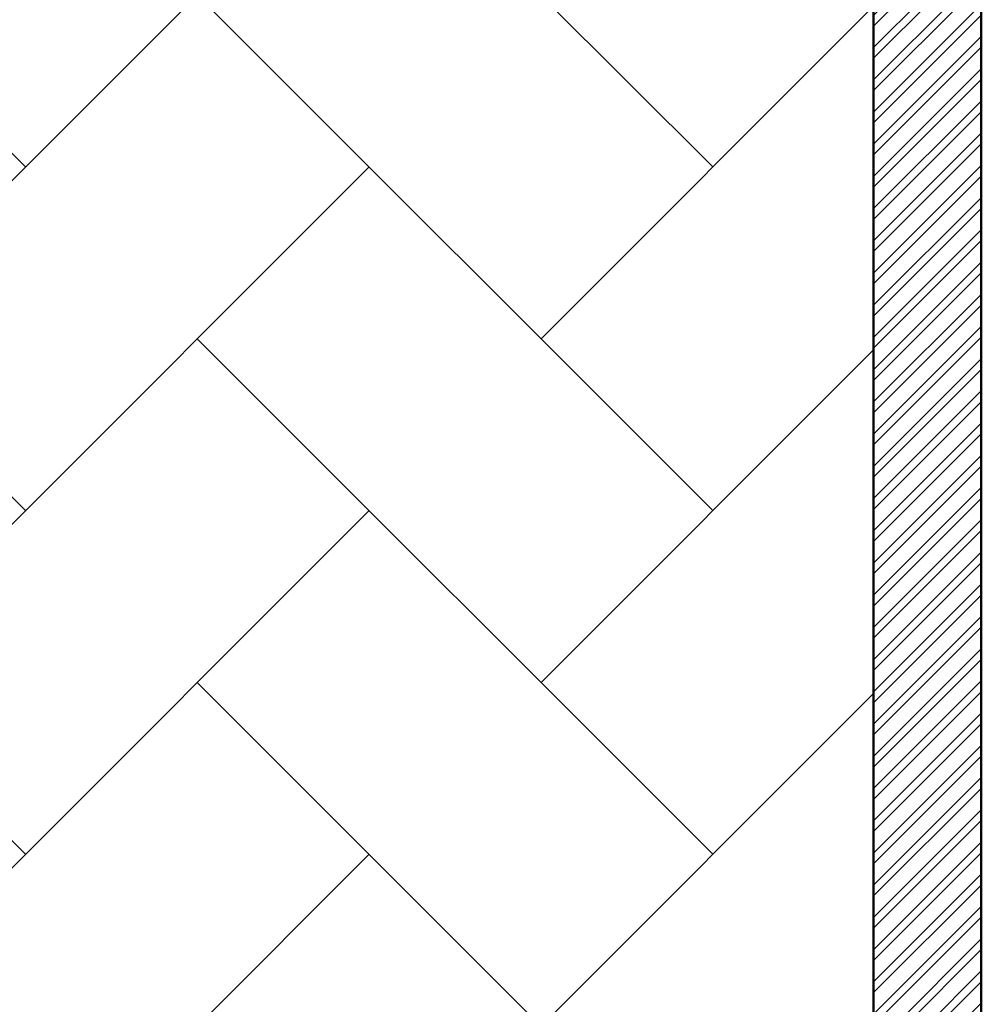
# Model space of a CAD drawing. Units: inches. Extents: x 3590 to 5167, y 65 to 1917.
# Tile 68 of 100: x 5000 to 5080, y 1640 to 1722. Entities that reach past the tile are written whole.
import ezdxf

# ---------------------------------------------------------------- set-up
doc = ezdxf.new("R2010")
doc.units = ezdxf.units.IN
for name, color, linetype, lineweight in [('A-FLOR-PATT', 8, 'Continuous', 13), ('A-WALL', 7, 'Continuous', 50), ('A-WALL-PATT', 251, 'Continuous', 13)]:
    doc.layers.add(name, color=color, linetype=linetype, lineweight=lineweight)

msp = doc.modelspace()

# ---------------------------------------------------------------- hatches: boundary and pattern name
at = {"layer": 'A-FLOR-PATT', "transparency": 33554687}
h = msp.add_hatch(dxfattribs=at)
h.set_pattern_fill('AR-HBONE', color=256, scale=0.2)
h.set_pattern_definition([(45, (-588.972, 0), (0, 28.73682), [60.96, -20.32]), (135, (-574.604, 14.368), (3e-15, 28.73682), [60.96, -20.32])])
h.paths.add_polyline_path([(5071.274, 1796.999), (4933.274, 1796.999), (4933.274, 1753.999), (4962.774, 1753.999, -0.414214), (4928.774, 1719.999), (4933.274, 1718.999), (4933.274, 1334.999), (5071.274, 1334.999)])
h.paths.add_polyline_path([(4951.78, 1521.077), (4951.715, 1521.04), (4951.563, 1520.895)], flags=16)
h.paths.add_polyline_path([(4952.267, 1521.376), (4952.198, 1521.371), (4952.198, 1521.356)], flags=0)
h.paths.add_polyline_path([(4967.051, 1529.728), (4965.231, 1528.694), (4963.411, 1527.714), (4961.756, 1526.851), (4963.589, 1527.449), (4964.036, 1527.478), (4962.975, 1527.249), (4961.76, 1526.852), (4959.792, 1525.834), (4958.005, 1524.895), (4956.24, 1523.93), (4954.504, 1522.919), (4954.129, 1522.682), (4953.361, 1521.997), (4953.366, 1521.998), (4953.605, 1522.064), (4955.106, 1522.761), (4956.921, 1523.434), (4958.678, 1523.915), (4960.358, 1524.2), (4961.945, 1524.286), (4964.171, 1524.108), (4965.958, 1523.309), (4963.863, 1522.976), (4965.187, 1522.499), (4963.366, 1522.497), (4961.545, 1522.487), (4959.764, 1522.461), (4958.304, 1522.419), (4957.974, 1522.388), (4956.307, 1522.232), (4954.718, 1522.071), (4953.251, 1521.899), (4953.525, 1521.623), (4954.331, 1521.379), (4956.243, 1521.23), (4958.039, 1520.93), (4959.684, 1520.483), (4961.16, 1519.896), (4963.107, 1518.8), (4964.393, 1517.325), (4962.973, 1517.726), (4964.558, 1516.661), (4965.407, 1515.708), (4963.507, 1516.322), (4961.68, 1517.005), (4959.935, 1517.745), (4958.282, 1518.528), (4956.732, 1519.343), (4955.295, 1520.175), (4954.672, 1520.572), (4954.513, 1520.627), (4955.658, 1519.318), (4956.703, 1517.982), (4957.644, 1516.647), (4958.485, 1515.334), (4959.55, 1513.524), (4960.438, 1511.769), (4958.841, 1513.62), (4957.452, 1515.325), (4955.819, 1517.459), (4956.665, 1515.448), (4957.111, 1513.923), (4957.447, 1511.714), (4957.076, 1509.793), (4956.538, 1511.11), (4955.992, 1512.569), (4955.444, 1514.125), (4954.898, 1515.735), (4954.357, 1517.356), (4953.824, 1518.943), (4953.305, 1520.452), (4953.065, 1521.116), (4952.971, 1521.146), (4952.949, 1521.086), (4952.73, 1520.199), (4953.37, 1518.024), (4953.757, 1516.373), (4954.051, 1514.765), (4954.264, 1513.221), (4954.471, 1511.131), (4954.497, 1510.402), (4954.409, 1511.76), (4954.264, 1513.221), (4954.051, 1514.765), (4953.757, 1516.373), (4953.37, 1518.024), (4952.877, 1519.698), (4952.716, 1520.141), (4952.533, 1519.059), (4952.374, 1517.789), (4952.219, 1516.312), (4952.046, 1514.6), (4951.833, 1512.626), (4951.557, 1510.363), (4951.203, 1512.168), (4950.852, 1514.339), (4950.985, 1516.376), (4951.66, 1518.286), (4952.593, 1520.481), (4952.357, 1521.13), (4951.855, 1520.328), (4950.839, 1518.908), (4949.777, 1517.587), (4948.916, 1516.617), (4948.111, 1515.256), (4947.089, 1513.554), (4945.889, 1511.615), (4946.326, 1513.402), (4946.562, 1514.249), (4945.528, 1513.327), (4944.581, 1512.531), (4946.018, 1514.508), (4947.204, 1516.048), (4947.893, 1517.313), (4949.307, 1518.764), (4950.414, 1519.767), (4950.451, 1519.806), (4952.267, 1521.376), (4951.645, 1521.493), (4950.404, 1521.18), (4948.044, 1520.359), (4946.119, 1519.452), (4944.572, 1518.475), (4943.35, 1517.443), (4941.997, 1515.92), (4941.661, 1515.275), (4942.813, 1516.99), (4944.572, 1518.475), (4946.119, 1519.452), (4948.044, 1520.359), (4950.404, 1521.18), (4951.645, 1521.493), (4949.647, 1521.868), (4948.6, 1521.756), (4947.126, 1521.57), (4945.42, 1521.348), (4943.45, 1521.105), (4941.183, 1520.856), (4942.86, 1521.613), (4943.873, 1522.03), (4942.952, 1521.909), (4941.41, 1521.485), (4939.543, 1520.67), (4938.968, 1520.226), (4940.733, 1521.299), (4942.952, 1521.909), (4943.702, 1522.008), (4945.894, 1522.7), (4947.565, 1522.714), (4948.921, 1522.566), (4951.131, 1522.183), (4950.971, 1522.297), (4948.129, 1523.006), (4946.035, 1523.707), (4944.232, 1524.521), (4942.707, 1525.461), (4941.444, 1526.537), (4940.43, 1527.761), (4939.649, 1529.143), (4941.421, 1528.122), (4943.147, 1527.132), (4944.841, 1526.175), (4946.514, 1525.25), (4948.179, 1524.359), (4948.365, 1524.263), (4946.475, 1526.045), (4945.181, 1527.54), (4944.19, 1529.033), (4943.496, 1530.54), (4943.278, 1531.36), (4942.498, 1531.919), (4943.114, 1531.762), (4942.959, 1533.659), (4944.14, 1531.989), (4944.612, 1531.323), (4946.202, 1530.463), (4947.486, 1529.509), (4948.79, 1528.226), (4950.368, 1526.237), (4949.485, 1528.155), (4948.851, 1530.123), (4948.491, 1532.041), (4948.381, 1533.918), (4948.501, 1535.76), (4948.827, 1537.573), (4949.418, 1535.565), (4949.957, 1533.569), (4950.464, 1531.586), (4950.961, 1529.617), (4951.391, 1527.954), (4951.724, 1530.687), (4952.201, 1532.58), (4952.889, 1534.33), (4953.77, 1535.951), (4954.827, 1537.46), (4954.521, 1535.39), (4954.273, 1533.937), (4955.58, 1535.663), (4956.748, 1536.739), (4956.159, 1534.78), (4955.589, 1532.873), (4955.043, 1531.006), (4954.525, 1529.166), (4954.038, 1527.341), (4953.638, 1525.733), (4953.611, 1525.586), (4953.398, 1524.166), (4953.382, 1524.009), (4954.07, 1525.476), (4954.912, 1527.022), (4956.136, 1528.894), (4957.847, 1530.577), (4959.376, 1531.54), (4958.256, 1530.104), (4957.143, 1528.663), (4956.066, 1527.243), (4955.056, 1525.871), (4954.141, 1524.571), (4953.352, 1523.372), (4953.311, 1523.303), (4953.273, 1522.925), (4953.261, 1522.382), (4954.103, 1523.373), (4954.63, 1524.284), (4955.961, 1526.358), (4957.23, 1528.13), (4958.421, 1529.609), (4960.037, 1531.368), (4961.374, 1532.375), (4962.101, 1532.77), (4961.07, 1531.061), (4959.987, 1529.438), (4958.869, 1527.908), (4958.15, 1527.007), (4959.803, 1528.003), (4961.589, 1528.793), (4963.391, 1529.328), (4965.211, 1529.632)], flags=16)
h.paths.add_polyline_path([(4962.944, 1523.182), (4961.107, 1523.422), (4960.392, 1523.362), (4962.35, 1523.331)], flags=0)
h.paths.add_polyline_path([(5049.541, 1584.551), (5049.476, 1584.515), (5049.325, 1584.37)], flags=16)
h.paths.add_polyline_path([(5050.028, 1584.851), (5049.959, 1584.845), (5049.959, 1584.83)], flags=0)
h.paths.add_polyline_path([(5042.333, 1581.949), (5043.88, 1582.926), (5045.806, 1583.833), (5048.165, 1584.654), (5049.406, 1584.967), (5047.408, 1585.342), (5046.361, 1585.231), (5044.888, 1585.044), (5043.181, 1584.822), (5041.211, 1584.579), (5038.944, 1584.33), (5040.622, 1585.087), (5041.634, 1585.504), (5040.713, 1585.383), (5039.171, 1584.959), (5037.304, 1584.144), (5036.729, 1583.7), (5038.494, 1584.773), (5040.713, 1585.383), (5041.463, 1585.482), (5043.655, 1586.174), (5045.326, 1586.188), (5046.682, 1586.04), (5048.893, 1585.657), (5048.732, 1585.771), (5045.891, 1586.48), (5043.796, 1587.181), (5041.994, 1587.996), (5040.468, 1588.935), (5039.205, 1590.011), (5038.191, 1591.235), (5037.41, 1592.617), (5039.182, 1591.596), (5040.909, 1590.607), (5042.602, 1589.649), (5044.275, 1588.724), (5045.94, 1587.833), (5046.126, 1587.738), (5044.237, 1589.519), (5042.942, 1591.015), (5041.952, 1592.508), (5041.257, 1594.014), (5041.039, 1594.834), (5040.26, 1595.393), (5040.875, 1595.237), (5040.721, 1597.133), (5041.901, 1595.463), (5042.373, 1594.798), (5043.963, 1593.938), (5045.247, 1592.983), (5046.552, 1591.701), (5048.129, 1589.712), (5047.247, 1591.63), (5046.613, 1593.597), (5046.252, 1595.515), (5046.142, 1597.392), (5046.262, 1599.234), (5046.588, 1601.047), (5047.179, 1599.039), (5047.718, 1597.043), (5048.225, 1595.06), (5048.722, 1593.091), (5049.152, 1591.429), (5049.485, 1594.161), (5049.962, 1596.054), (5050.65, 1597.804), (5051.532, 1599.425), (5052.589, 1600.934), (5052.283, 1598.864), (5052.034, 1597.411), (5053.341, 1599.137), (5054.509, 1600.213), (5053.92, 1598.254), (5053.35, 1596.348), (5052.805, 1594.48), (5052.286, 1592.64), (5051.799, 1590.815), (5051.4, 1589.207), (5051.373, 1589.06), (5051.159, 1587.64), (5051.143, 1587.483), (5051.831, 1588.95), (5052.673, 1590.496), (5053.898, 1592.368), (5055.608, 1594.051), (5057.137, 1595.014), (5056.017, 1593.578), (5054.904, 1592.137), (5053.828, 1590.717), (5052.817, 1589.345), (5051.902, 1588.046), (5051.113, 1586.846), (5051.072, 1586.777), (5051.034, 1586.399), (5051.022, 1585.856), (5051.864, 1586.847), (5052.391, 1587.758), (5053.723, 1589.832), (5054.991, 1591.604), (5056.182, 1593.083), (5057.798, 1594.842), (5059.135, 1595.849), (5059.863, 1596.244), (5058.831, 1594.535), (5057.749, 1592.912), (5056.63, 1591.382), (5055.912, 1590.482), (5057.564, 1591.477), (5059.35, 1592.267), (5061.152, 1592.802), (5062.972, 1593.106), (5064.812, 1593.203), (5062.992, 1592.169), (5061.172, 1591.188), (5059.518, 1590.325), (5061.35, 1590.924), (5061.797, 1590.952), (5060.737, 1590.723), (5059.521, 1590.326), (5057.553, 1589.308), (5055.766, 1588.369), (5054.002, 1587.404), (5052.265, 1586.393), (5051.891, 1586.156), (5051.122, 1585.471), (5051.127, 1585.472), (5051.366, 1585.538), (5052.867, 1586.235), (5054.682, 1586.908), (5056.439, 1587.389), (5058.12, 1587.675), (5059.706, 1587.76), (5061.933, 1587.583), (5063.719, 1586.783), (5061.624, 1586.45), (5062.949, 1585.973), (5061.127, 1585.971), (5059.307, 1585.961), (5057.525, 1585.935), (5056.065, 1585.893), (5055.735, 1585.862), (5054.068, 1585.707), (5052.479, 1585.546), (5051.012, 1585.373), (5051.286, 1585.097), (5052.092, 1584.853), (5054.004, 1584.704), (5055.8, 1584.404), (5057.446, 1583.958), (5058.921, 1583.37), (5060.868, 1582.274), (5062.154, 1580.799), (5060.734, 1581.2), (5062.32, 1580.135), (5063.168, 1579.182), (5061.269, 1579.796), (5059.441, 1580.479), (5057.696, 1581.219), (5056.043, 1582.003), (5054.493, 1582.817), (5053.057, 1583.649), (5052.433, 1584.047), (5052.274, 1584.101), (5053.42, 1582.793), (5054.464, 1581.457), (5055.405, 1580.121), (5056.247, 1578.809), (5057.311, 1576.998), (5058.199, 1575.244), (5056.602, 1577.094), (5055.213, 1578.799), (5053.58, 1580.933), (5054.427, 1578.922), (5054.872, 1577.397), (5055.208, 1575.189), (5054.838, 1573.267), (5054.299, 1574.584), (5053.754, 1576.043), (5053.206, 1577.599), (5052.659, 1579.209), (5052.118, 1580.83), (5051.585, 1582.417), (5051.066, 1583.927), (5050.826, 1584.59), (5050.733, 1584.62), (5050.711, 1584.561), (5050.491, 1583.673), (5051.131, 1581.498), (5051.518, 1579.847), (5051.813, 1578.24), (5052.026, 1576.695), (5052.233, 1574.605), (5052.258, 1573.876), (5052.17, 1575.234), (5052.026, 1576.695), (5051.813, 1578.24), (5051.518, 1579.847), (5051.131, 1581.498), (5050.638, 1583.172), (5050.477, 1583.615), (5050.294, 1582.533), (5050.136, 1581.263), (5049.981, 1579.786), (5049.807, 1578.074), (5049.594, 1576.1), (5049.318, 1573.837), (5048.965, 1575.642), (5048.613, 1577.813), (5048.747, 1579.85), (5049.421, 1581.76), (5050.354, 1583.955), (5050.118, 1584.604), (5049.616, 1583.802), (5048.6, 1582.382), (5047.538, 1581.061), (5046.677, 1580.091), (5045.872, 1578.73), (5044.85, 1577.028), (5043.651, 1575.089), (5044.087, 1576.877), (5044.324, 1577.723), (5043.289, 1576.801), (5042.342, 1576.005), (5043.779, 1577.982), (5044.966, 1579.522), (5045.655, 1580.787), (5047.068, 1582.239), (5048.175, 1583.241), (5048.213, 1583.28), (5050.028, 1584.851), (5049.406, 1584.967), (5048.165, 1584.654), (5045.806, 1583.833), (5043.88, 1582.926), (5042.333, 1581.949), (5041.111, 1580.917), (5039.758, 1579.394), (5039.423, 1578.749), (5040.575, 1580.464)], flags=16)
h.paths.add_polyline_path([(4954.799, 1533.12), (4954.262, 1532.079), (4953.831, 1530.935), (4953.505, 1529.636), (4953.283, 1528.133), (4953.167, 1526.376), (4953.156, 1524.315), (4953.277, 1521.236), (4952.802, 1521.842), (4951.557, 1521.998), (4950.976, 1521.961), (4952.661, 1521.941), (4952.802, 1521.842), (4953.152, 1523.593), (4953.167, 1526.376), (4953.283, 1528.133), (4953.609, 1530.346), (4954.456, 1532.592)], flags=0)
h.paths.add_polyline_path([(5050.563, 1585.316), (5049.318, 1585.472), (5048.737, 1585.435), (5050.422, 1585.415), (5050.563, 1585.316), (5050.914, 1587.067), (5050.928, 1589.851), (5051.045, 1591.607), (5051.371, 1593.82), (5052.217, 1596.066), (5052.56, 1596.594), (5052.024, 1595.554), (5051.592, 1594.409), (5051.266, 1593.11), (5051.045, 1591.607), (5050.928, 1589.851), (5050.918, 1587.789), (5051.038, 1584.71)], flags=0)
h.paths.add_polyline_path([(5058.153, 1586.836), (5060.111, 1586.805), (5060.705, 1586.656), (5058.868, 1586.896)], flags=0)
h.paths.add_polyline_path([(5049.541, 1430.936), (5049.476, 1430.9), (5049.325, 1430.755)], flags=16)
h.paths.add_polyline_path([(5050.028, 1431.236), (5049.959, 1431.231), (5049.959, 1431.215)], flags=0)
h.paths.add_polyline_path([(5046.588, 1447.432), (5047.179, 1445.425), (5047.718, 1443.429), (5048.225, 1441.446), (5048.722, 1439.476), (5049.152, 1437.814), (5049.485, 1440.546), (5049.962, 1442.439), (5050.65, 1444.189), (5051.532, 1445.811), (5052.589, 1447.319), (5052.283, 1445.249), (5052.034, 1443.796), (5053.341, 1445.522), (5054.509, 1446.598), (5053.92, 1444.64), (5053.35, 1442.733), (5052.805, 1440.865), (5052.286, 1439.025), (5051.799, 1437.201), (5051.4, 1435.592), (5051.373, 1435.445), (5051.159, 1434.025), (5051.143, 1433.868), (5051.831, 1435.335), (5052.673, 1436.881), (5053.898, 1438.753), (5055.608, 1440.436), (5057.137, 1441.4), (5056.017, 1439.963), (5054.904, 1438.522), (5053.828, 1437.102), (5052.817, 1435.73), (5051.902, 1434.431), (5051.113, 1433.231), (5051.072, 1433.162), (5051.034, 1432.784), (5051.022, 1432.242), (5051.864, 1433.232), (5052.391, 1434.143), (5053.723, 1436.217), (5054.991, 1437.989), (5056.182, 1439.468), (5057.798, 1441.227), (5059.135, 1442.235), (5059.863, 1442.629), (5058.831, 1440.921), (5057.749, 1439.298), (5056.63, 1437.767), (5055.912, 1436.867), (5057.564, 1437.863), (5059.35, 1438.652), (5061.152, 1439.187), (5062.972, 1439.491), (5064.812, 1439.588), (5062.992, 1438.554), (5061.172, 1437.573), (5059.518, 1436.71), (5061.35, 1437.309), (5061.797, 1437.337), (5060.737, 1437.108), (5059.521, 1436.711), (5057.553, 1435.693), (5055.766, 1434.754), (5054.002, 1433.789), (5052.265, 1432.778), (5051.891, 1432.541), (5051.122, 1431.856), (5051.127, 1431.857), (5051.366, 1431.923), (5052.867, 1432.62), (5054.682, 1433.293), (5056.439, 1433.775), (5058.12, 1434.06), (5059.706, 1434.145), (5061.933, 1433.968), (5063.719, 1433.168), (5061.624, 1432.835), (5062.949, 1432.358), (5061.127, 1432.357), (5059.307, 1432.346), (5057.525, 1432.32), (5056.065, 1432.278), (5055.735, 1432.248), (5054.068, 1432.092), (5052.479, 1431.931), (5051.012, 1431.759), (5051.286, 1431.482), (5052.092, 1431.238), (5054.004, 1431.089), (5055.8, 1430.789), (5057.446, 1430.343), (5058.921, 1429.755), (5060.868, 1428.66), (5062.154, 1427.185), (5060.734, 1427.585), (5062.32, 1426.52), (5063.168, 1425.567), (5061.269, 1426.181), (5059.441, 1426.865), (5057.696, 1427.604), (5056.043, 1428.388), (5054.493, 1429.202), (5053.057, 1430.034), (5052.433, 1430.432), (5052.274, 1430.487), (5053.42, 1429.178), (5054.464, 1427.842), (5055.405, 1426.506), (5056.247, 1425.194), (5057.311, 1423.383), (5058.199, 1421.629), (5056.602, 1423.479), (5055.213, 1425.184), (5053.58, 1427.318), (5054.427, 1425.307), (5054.872, 1423.782), (5055.208, 1421.574), (5054.838, 1419.652), (5054.299, 1420.97), (5053.754, 1422.428), (5053.206, 1423.984), (5052.659, 1425.595), (5052.118, 1427.215), (5051.585, 1428.802), (5051.066, 1430.312), (5050.826, 1430.975), (5050.733, 1431.005), (5050.711, 1430.946), (5050.491, 1430.058), (5051.131, 1427.883), (5051.518, 1426.232), (5051.813, 1424.625), (5052.026, 1423.081), (5052.233, 1420.991), (5052.258, 1420.261), (5052.17, 1421.619), (5052.026, 1423.081), (5051.813, 1424.625), (5051.518, 1426.232), (5051.131, 1427.883), (5050.638, 1429.558), (5050.477, 1430.001), (5050.294, 1428.918), (5050.136, 1427.648), (5049.981, 1426.171), (5049.807, 1424.459), (5049.594, 1422.485), (5049.318, 1420.222), (5048.965, 1422.028), (5048.613, 1424.199), (5048.747, 1426.235), (5049.421, 1428.146), (5050.354, 1430.34), (5050.118, 1430.989), (5049.616, 1430.187), (5048.6, 1428.768), (5047.538, 1427.446), (5046.677, 1426.477), (5045.872, 1425.116), (5044.85, 1423.413), (5043.651, 1421.474), (5044.087, 1423.262), (5044.324, 1424.109), (5043.289, 1423.186), (5042.342, 1422.391), (5043.779, 1424.368), (5044.966, 1425.907), (5045.655, 1427.173), (5047.068, 1428.624), (5048.175, 1429.627), (5048.213, 1429.666), (5050.028, 1431.236), (5049.406, 1431.353), (5048.165, 1431.039), (5045.806, 1430.218), (5043.88, 1429.311), (5042.333, 1428.334), (5041.111, 1427.302), (5039.758, 1425.779), (5039.423, 1425.134), (5040.575, 1426.849), (5042.333, 1428.334), (5043.88, 1429.311), (5045.806, 1430.218), (5048.165, 1431.039), (5049.406, 1431.353), (5047.408, 1431.727), (5046.361, 1431.616), (5044.888, 1431.429), (5043.181, 1431.207), (5041.211, 1430.964), (5038.944, 1430.715), (5040.622, 1431.472), (5041.634, 1431.89), (5040.713, 1431.769), (5039.171, 1431.345), (5037.304, 1430.53), (5036.729, 1430.085), (5038.494, 1431.158), (5040.713, 1431.769), (5041.463, 1431.867), (5043.655, 1432.559), (5045.326, 1432.573), (5046.682, 1432.425), (5048.893, 1432.042), (5048.732, 1432.156), (5045.891, 1432.865), (5043.796, 1433.566), (5041.994, 1434.381), (5040.468, 1435.321), (5039.205, 1436.396), (5038.191, 1437.62), (5037.41, 1439.002), (5039.182, 1437.982), (5040.909, 1436.992), (5042.602, 1436.034), (5044.275, 1435.109), (5045.94, 1434.218), (5046.126, 1434.123), (5044.237, 1435.904), (5042.942, 1437.4), (5041.952, 1438.893), (5041.257, 1440.399), (5041.039, 1441.219), (5040.26, 1441.778), (5040.875, 1441.622), (5040.721, 1443.518), (5041.901, 1441.848), (5042.373, 1441.183), (5043.963, 1440.323), (5045.247, 1439.369), (5046.552, 1438.086), (5048.129, 1436.097), (5047.247, 1438.015), (5046.613, 1439.982), (5046.252, 1441.901), (5046.142, 1443.778), (5046.262, 1445.619)], flags=16)
h.paths.add_polyline_path([(5052.382, 1444.255), (5051.623, 1442.78), (5052.024, 1441.939), (5052.56, 1442.98)], flags=0)
h.paths.add_polyline_path([(5050.563, 1431.701), (5049.318, 1431.857), (5048.737, 1431.821), (5050.422, 1431.8)], flags=0)
h.paths.add_polyline_path([(5058.153, 1433.221), (5060.111, 1433.19), (5060.705, 1433.041), (5058.868, 1433.281)], flags=0)
h.paths.add_polyline_path([(5049.541, 1352.285), (5049.476, 1352.249), (5049.325, 1352.104)], flags=16)
h.paths.add_polyline_path([(5050.028, 1352.585), (5049.959, 1352.58), (5049.959, 1352.564)], flags=0)
h.paths.add_polyline_path([(5046.588, 1368.781), (5047.179, 1366.774), (5047.718, 1364.778), (5048.225, 1362.795), (5048.722, 1360.825), (5049.152, 1359.163), (5049.485, 1361.896), (5049.962, 1363.789), (5050.65, 1365.538), (5051.532, 1367.16), (5052.589, 1368.669), (5052.283, 1366.598), (5052.034, 1365.145), (5053.341, 1366.871), (5054.509, 1367.947), (5053.92, 1365.989), (5053.35, 1364.082), (5052.805, 1362.214), (5052.286, 1360.374), (5051.799, 1358.55), (5051.4, 1356.942), (5051.373, 1356.794), (5051.159, 1355.374), (5051.143, 1355.218), (5051.831, 1356.684), (5052.673, 1358.23), (5053.898, 1360.102), (5055.608, 1361.786), (5057.137, 1362.749), (5056.017, 1361.313), (5054.904, 1359.872), (5053.828, 1358.452), (5052.817, 1357.079), (5051.902, 1355.78), (5051.113, 1354.581), (5051.072, 1354.512), (5051.034, 1354.133), (5051.022, 1353.591), (5051.864, 1354.581), (5052.391, 1355.492), (5053.723, 1357.566), (5054.991, 1359.338), (5056.182, 1360.817), (5057.798, 1362.577), (5059.135, 1363.584), (5059.863, 1363.979), (5058.831, 1362.27), (5057.749, 1360.647), (5056.63, 1359.117), (5055.912, 1358.216), (5057.564, 1359.212), (5059.35, 1360.001), (5061.152, 1360.536), (5062.972, 1360.841), (5064.812, 1360.937), (5062.992, 1359.903), (5061.172, 1358.923), (5059.518, 1358.059), (5061.35, 1358.658), (5061.797, 1358.687), (5060.737, 1358.458), (5059.521, 1358.061), (5057.553, 1357.043), (5055.766, 1356.103), (5054.002, 1355.138), (5052.265, 1354.127), (5051.891, 1353.89), (5051.122, 1353.206), (5051.127, 1353.206), (5051.366, 1353.272), (5052.867, 1353.969), (5054.682, 1354.643), (5056.439, 1355.124), (5058.12, 1355.409), (5059.706, 1355.495), (5061.933, 1355.317), (5063.719, 1354.518), (5061.624, 1354.184), (5062.949, 1353.708), (5061.127, 1353.706), (5059.307, 1353.695), (5057.525, 1353.669), (5056.065, 1353.627), (5055.735, 1353.597), (5054.068, 1353.441), (5052.479, 1353.28), (5051.012, 1353.108), (5051.286, 1352.831), (5052.092, 1352.587), (5054.004, 1352.439), (5055.8, 1352.138), (5057.446, 1351.692), (5058.921, 1351.104), (5060.868, 1350.009), (5062.154, 1348.534), (5060.734, 1348.935), (5062.32, 1347.869), (5063.168, 1346.916), (5061.269, 1347.53), (5059.441, 1348.214), (5057.696, 1348.954), (5056.043, 1349.737), (5054.493, 1350.551), (5053.057, 1351.383), (5052.433, 1351.781), (5052.274, 1351.836), (5053.42, 1350.527), (5054.464, 1349.191), (5055.405, 1347.855), (5056.247, 1346.543), (5057.311, 1344.733), (5058.199, 1342.978), (5056.602, 1344.828), (5055.213, 1346.534), (5053.58, 1348.667), (5054.427, 1346.656), (5054.872, 1345.132), (5055.208, 1342.923), (5054.838, 1341.002), (5054.299, 1342.319), (5053.754, 1343.778), (5053.206, 1345.334), (5052.659, 1346.944), (5052.118, 1348.564), (5051.585, 1350.151), (5051.066, 1351.661), (5050.826, 1352.324), (5050.733, 1352.355), (5050.711, 1352.295), (5050.491, 1351.408), (5051.131, 1349.232), (5051.518, 1347.581), (5051.813, 1345.974), (5052.026, 1344.43), (5052.233, 1342.34), (5052.258, 1341.61), (5052.17, 1342.969), (5052.026, 1344.43), (5051.813, 1345.974), (5051.518, 1347.581), (5051.131, 1349.232), (5050.638, 1350.907), (5050.477, 1351.35), (5050.294, 1350.267), (5050.136, 1348.997), (5049.981, 1347.52), (5049.807, 1345.809), (5049.594, 1343.835), (5049.318, 1341.571), (5048.965, 1343.377), (5048.613, 1345.548), (5048.747, 1347.585), (5049.421, 1349.495), (5050.354, 1351.689), (5050.118, 1352.339), (5049.616, 1351.536), (5048.6, 1350.117), (5047.538, 1348.795), (5046.677, 1347.826), (5045.872, 1346.465), (5044.85, 1344.763), (5043.651, 1342.824), (5044.087, 1344.611), (5044.324, 1345.458), (5043.289, 1344.535), (5042.342, 1343.74), (5043.779, 1345.717), (5044.966, 1347.256), (5045.655, 1348.522), (5047.068, 1349.973), (5048.175, 1350.976), (5048.213, 1351.015), (5050.028, 1352.585), (5049.406, 1352.702), (5048.165, 1352.388), (5045.806, 1351.567), (5043.88, 1350.661), (5042.333, 1349.683), (5041.111, 1348.651), (5039.758, 1347.128), (5039.423, 1346.483), (5040.575, 1348.198), (5042.333, 1349.683), (5043.88, 1350.661), (5045.806, 1351.567), (5048.165, 1352.388), (5049.406, 1352.702), (5047.408, 1353.076), (5046.361, 1352.965), (5044.888, 1352.779), (5043.181, 1352.556), (5041.211, 1352.313), (5038.944, 1352.065), (5040.622, 1352.821), (5041.634, 1353.239), (5040.713, 1353.118), (5039.171, 1352.694), (5037.304, 1351.879), (5036.729, 1351.434), (5038.494, 1352.508), (5040.713, 1353.118), (5041.463, 1353.216), (5043.655, 1353.909), (5045.326, 1353.923), (5046.682, 1353.774), (5048.893, 1353.391), (5048.732, 1353.506), (5045.891, 1354.214), (5043.796, 1354.915), (5041.994, 1355.73), (5040.468, 1356.67), (5039.205, 1357.746), (5038.191, 1358.969), (5037.41, 1360.352), (5039.182, 1359.331), (5040.909, 1358.341), (5042.602, 1357.383), (5044.275, 1356.458), (5045.94, 1355.567), (5046.126, 1355.472), (5044.237, 1357.253), (5042.942, 1358.749), (5041.952, 1360.242), (5041.257, 1361.748), (5041.039, 1362.568), (5040.26, 1363.128), (5040.875, 1362.971), (5040.721, 1364.867), (5041.901, 1363.197), (5042.373, 1362.532), (5043.963, 1361.672), (5045.247, 1360.718), (5046.552, 1359.435), (5048.129, 1357.446), (5047.247, 1359.364), (5046.613, 1361.331), (5046.252, 1363.25), (5046.142, 1365.127), (5046.262, 1366.969)], flags=16)
h.paths.add_polyline_path([(5052.382, 1365.604), (5051.623, 1364.129), (5052.024, 1363.288), (5052.56, 1364.329)], flags=0)
h.paths.add_polyline_path([(4951.78, 1698.041), (4951.715, 1698.005), (4951.563, 1697.859)], flags=16)
h.paths.add_polyline_path([(4952.267, 1698.341), (4952.198, 1698.335), (4952.198, 1698.32)], flags=0)
h.paths.add_polyline_path([(4957.076, 1686.757), (4956.538, 1688.074), (4955.992, 1689.533), (4955.444, 1691.089), (4954.898, 1692.699), (4954.357, 1694.32), (4953.824, 1695.907), (4953.305, 1697.417), (4953.065, 1698.08), (4952.971, 1698.11), (4952.949, 1698.051), (4952.73, 1697.163), (4953.37, 1694.988), (4953.757, 1693.337), (4954.051, 1691.729), (4954.264, 1690.185), (4954.471, 1688.095), (4954.497, 1687.366), (4954.409, 1688.724), (4954.264, 1690.185), (4954.051, 1691.729), (4953.757, 1693.337), (4953.37, 1694.988), (4952.877, 1696.662), (4952.716, 1697.105), (4952.533, 1696.023), (4952.374, 1694.753), (4952.219, 1693.276), (4952.046, 1691.564), (4951.833, 1689.59), (4951.557, 1687.327), (4951.203, 1689.132), (4950.852, 1691.303), (4950.985, 1693.34), (4951.66, 1695.25), (4952.593, 1697.445), (4952.357, 1698.094), (4951.855, 1697.292), (4950.839, 1695.872), (4949.777, 1694.551), (4948.916, 1693.581), (4948.111, 1692.22), (4947.089, 1690.518), (4945.889, 1688.579), (4946.326, 1690.366), (4946.562, 1691.213), (4945.528, 1690.291), (4944.581, 1689.495), (4946.018, 1691.472), (4947.204, 1693.012), (4947.893, 1694.277), (4949.307, 1695.729), (4950.414, 1696.731), (4950.451, 1696.77), (4952.267, 1698.341), (4951.645, 1698.457), (4950.404, 1698.144), (4948.044, 1697.323), (4946.119, 1696.416), (4944.572, 1695.439), (4943.35, 1694.407), (4941.997, 1692.884), (4941.661, 1692.239), (4942.813, 1693.954), (4944.572, 1695.439), (4946.119, 1696.416), (4948.044, 1697.323), (4950.404, 1698.144), (4951.645, 1698.457), (4949.647, 1698.832), (4948.6, 1698.72), (4947.126, 1698.534), (4945.42, 1698.312), (4943.45, 1698.069), (4941.183, 1697.82), (4942.86, 1698.577), (4943.873, 1698.994), (4942.952, 1698.873), (4941.41, 1698.449), (4939.543, 1697.634), (4938.968, 1697.19), (4940.733, 1698.263), (4942.952, 1698.873), (4943.702, 1698.972), (4945.894, 1699.664), (4947.565, 1699.678), (4948.921, 1699.53), (4951.131, 1699.147), (4950.971, 1699.261), (4948.129, 1699.97), (4946.035, 1700.671), (4944.232, 1701.486), (4942.707, 1702.425), (4941.444, 1703.501), (4940.43, 1704.725), (4939.649, 1706.107), (4941.421, 1705.086), (4943.147, 1704.097), (4944.841, 1703.139), (4946.514, 1702.214), (4948.179, 1701.323), (4948.365, 1701.227), (4946.475, 1703.009), (4945.181, 1704.505), (4944.19, 1705.997), (4943.496, 1707.504), (4943.278, 1708.324), (4942.498, 1708.883), (4943.114, 1708.727), (4942.959, 1710.623), (4944.14, 1708.953), (4944.612, 1708.287), (4946.202, 1707.428), (4947.486, 1706.473), (4948.79, 1705.191), (4950.368, 1703.202), (4949.485, 1705.12), (4948.851, 1707.087), (4948.491, 1709.005), (4948.381, 1710.882), (4948.501, 1712.724), (4948.827, 1714.537), (4949.418, 1712.529), (4949.957, 1710.533), (4950.464, 1708.55), (4950.961, 1706.581), (4951.391, 1704.919), (4951.724, 1707.651), (4952.201, 1709.544), (4952.889, 1711.294), (4953.77, 1712.915), (4954.827, 1714.424), (4954.521, 1712.354), (4954.273, 1710.901), (4955.58, 1712.627), (4956.748, 1713.703), (4956.159, 1711.744), (4955.589, 1709.837), (4955.043, 1707.97), (4954.525, 1706.13), (4954.038, 1704.305), (4953.638, 1702.697), (4953.611, 1702.55), (4953.398, 1701.13), (4953.382, 1700.973), (4954.07, 1702.44), (4954.912, 1703.986), (4956.136, 1705.858), (4957.847, 1707.541), (4959.376, 1708.504), (4958.256, 1707.068), (4957.143, 1705.627), (4956.066, 1704.207), (4955.056, 1702.835), (4954.141, 1701.536), (4953.352, 1700.336), (4953.311, 1700.267), (4953.273, 1699.889), (4953.261, 1699.346), (4954.103, 1700.337), (4954.63, 1701.248), (4955.961, 1703.322), (4957.23, 1705.094), (4958.421, 1706.573), (4960.037, 1708.332), (4961.374, 1709.339), (4962.101, 1709.734), (4961.07, 1708.025), (4959.987, 1706.402), (4958.869, 1704.872), (4958.15, 1703.972), (4959.803, 1704.967), (4961.589, 1705.757), (4963.391, 1706.292), (4965.211, 1706.596), (4967.051, 1706.692), (4965.231, 1705.659), (4963.411, 1704.678), (4961.756, 1703.815), (4963.589, 1704.413), (4964.036, 1704.442), (4962.975, 1704.213), (4961.76, 1703.816), (4959.792, 1702.798), (4958.005, 1701.859), (4956.24, 1700.894), (4954.504, 1699.883), (4954.129, 1699.646), (4953.361, 1698.961), (4953.366, 1698.962), (4953.605, 1699.028), (4955.106, 1699.725), (4956.921, 1700.398), (4958.678, 1700.879), (4960.358, 1701.164), (4961.945, 1701.25), (4964.171, 1701.073), (4965.958, 1700.273), (4963.863, 1699.94), (4965.187, 1699.463), (4963.366, 1699.461), (4961.545, 1699.451), (4959.764, 1699.425), (4958.304, 1699.383), (4957.974, 1699.352), (4956.307, 1699.197), (4954.718, 1699.036), (4953.251, 1698.863), (4953.525, 1698.587), (4954.331, 1698.343), (4956.243, 1698.194), (4958.039, 1697.894), (4959.684, 1697.447), (4961.16, 1696.86), (4963.107, 1695.764), (4964.393, 1694.289), (4962.973, 1694.69), (4964.558, 1693.625), (4965.407, 1692.672), (4963.507, 1693.286), (4961.68, 1693.969), (4959.935, 1694.709), (4958.282, 1695.492), (4956.732, 1696.307), (4955.295, 1697.139), (4954.672, 1697.536), (4954.513, 1697.591), (4955.658, 1696.282), (4956.703, 1694.946), (4957.644, 1693.611), (4958.485, 1692.298), (4959.55, 1690.488), (4960.438, 1688.733), (4958.841, 1690.584), (4957.452, 1692.289), (4955.819, 1694.423), (4956.665, 1692.412), (4957.111, 1690.887), (4957.447, 1688.678)], flags=16)
h.paths.add_polyline_path([(5050.563, 1353.05), (5049.318, 1353.207), (5048.737, 1353.17), (5050.422, 1353.15)], flags=0)
h.paths.add_polyline_path([(4951.78, 1351.486), (4951.715, 1351.45), (4951.563, 1351.305)], flags=16)
h.paths.add_polyline_path([(4952.267, 1351.786), (4952.198, 1351.78), (4952.198, 1351.765)], flags=0)
h.paths.add_polyline_path([(4954.827, 1367.869), (4954.521, 1365.799), (4954.273, 1364.346), (4955.58, 1366.072), (4956.748, 1367.148), (4956.159, 1365.19), (4955.589, 1363.283), (4955.043, 1361.415), (4954.525, 1359.575), (4954.038, 1357.751), (4953.638, 1356.142), (4953.611, 1355.995), (4953.398, 1354.575), (4953.382, 1354.418), (4954.07, 1355.885), (4954.912, 1357.431), (4956.136, 1359.303), (4957.847, 1360.986), (4959.376, 1361.95), (4958.256, 1360.513), (4957.143, 1359.072), (4956.066, 1357.652), (4955.056, 1356.28), (4954.141, 1354.981), (4953.352, 1353.781), (4953.311, 1353.712), (4953.273, 1353.334), (4953.261, 1352.792), (4954.103, 1353.782), (4954.63, 1354.693), (4955.961, 1356.767), (4957.23, 1358.539), (4958.421, 1360.018), (4960.037, 1361.777), (4961.374, 1362.785), (4962.101, 1363.179), (4961.07, 1361.471), (4959.987, 1359.848), (4958.869, 1358.317), (4958.15, 1357.417), (4959.803, 1358.413), (4961.589, 1359.202), (4963.391, 1359.737), (4965.211, 1360.041), (4967.051, 1360.138), (4965.231, 1359.104), (4963.411, 1358.123), (4961.756, 1357.26), (4963.589, 1357.859), (4964.036, 1357.887), (4962.975, 1357.658), (4961.76, 1357.261), (4959.792, 1356.243), (4958.005, 1355.304), (4956.24, 1354.339), (4954.504, 1353.328), (4954.129, 1353.091), (4953.361, 1352.406), (4953.366, 1352.407), (4953.605, 1352.473), (4955.106, 1353.17), (4956.921, 1353.843), (4958.678, 1354.325), (4960.358, 1354.61), (4961.945, 1354.695), (4964.171, 1354.518), (4965.958, 1353.718), (4963.863, 1353.385), (4965.187, 1352.908), (4963.366, 1352.907), (4961.545, 1352.896), (4959.764, 1352.87), (4958.304, 1352.828), (4957.974, 1352.798), (4956.307, 1352.642), (4954.718, 1352.481), (4953.251, 1352.309), (4953.525, 1352.032), (4954.331, 1351.788), (4956.243, 1351.639), (4958.039, 1351.339), (4959.684, 1350.893), (4961.16, 1350.305), (4963.107, 1349.21), (4964.393, 1347.735), (4962.973, 1348.135), (4964.558, 1347.07), (4965.407, 1346.117), (4963.507, 1346.731), (4961.68, 1347.414), (4959.935, 1348.154), (4958.282, 1348.938), (4956.732, 1349.752), (4955.295, 1350.584), (4954.672, 1350.982), (4954.513, 1351.036), (4955.658, 1349.728), (4956.703, 1348.392), (4957.644, 1347.056), (4958.485, 1345.744), (4959.55, 1343.933), (4960.438, 1342.179), (4958.841, 1344.029), (4957.452, 1345.734), (4955.819, 1347.868), (4956.665, 1345.857), (4957.111, 1344.332), (4957.447, 1342.124), (4957.076, 1340.202), (4956.538, 1341.52), (4955.992, 1342.978), (4955.444, 1344.534), (4954.898, 1346.145), (4954.357, 1347.765), (4953.824, 1349.352), (4953.305, 1350.862), (4953.065, 1351.525), (4952.971, 1351.555), (4952.949, 1351.496), (4952.73, 1350.608), (4953.37, 1348.433), (4953.757, 1346.782), (4954.051, 1345.175), (4954.264, 1343.631), (4954.471, 1341.541), (4954.497, 1340.811), (4954.409, 1342.169), (4954.264, 1343.631), (4954.051, 1345.175), (4953.757, 1346.782), (4953.37, 1348.433), (4952.877, 1350.108), (4952.716, 1350.551), (4952.533, 1349.468), (4952.374, 1348.198), (4952.219, 1346.721), (4952.046, 1345.009), (4951.833, 1343.035), (4951.557, 1340.772), (4951.203, 1342.578), (4950.852, 1344.749), (4950.985, 1346.785), (4951.66, 1348.696), (4952.593, 1350.89), (4952.357, 1351.539), (4951.855, 1350.737), (4950.839, 1349.318), (4949.777, 1347.996), (4948.916, 1347.027), (4948.111, 1345.665), (4947.089, 1343.963), (4945.889, 1342.024), (4946.326, 1343.812), (4946.562, 1344.659), (4945.528, 1343.736), (4944.581, 1342.941), (4946.018, 1344.918), (4947.204, 1346.457), (4947.893, 1347.723), (4949.307, 1349.174), (4950.414, 1350.177), (4950.451, 1350.216), (4952.267, 1351.786), (4951.645, 1351.903), (4950.404, 1351.589), (4948.044, 1350.768), (4946.119, 1349.861), (4944.572, 1348.884), (4943.35, 1347.852), (4941.997, 1346.329), (4941.661, 1345.684), (4942.813, 1347.399), (4944.572, 1348.884), (4946.119, 1349.861), (4948.044, 1350.768), (4950.404, 1351.589), (4951.645, 1351.903), (4949.647, 1352.277), (4948.6, 1352.166), (4947.126, 1351.979), (4945.42, 1351.757), (4943.45, 1351.514), (4941.183, 1351.265), (4942.86, 1352.022), (4943.873, 1352.44), (4942.952, 1352.319), (4941.41, 1351.895), (4939.543, 1351.08), (4938.968, 1350.635), (4940.733, 1351.708), (4942.952, 1352.319), (4943.702, 1352.417), (4945.894, 1353.109), (4947.565, 1353.123), (4948.921, 1352.975), (4951.131, 1352.592), (4950.971, 1352.706), (4948.129, 1353.415), (4946.035, 1354.116), (4944.232, 1354.931), (4942.707, 1355.871), (4941.444, 1356.946), (4940.43, 1358.17), (4939.649, 1359.552), (4941.421, 1358.532), (4943.147, 1357.542), (4944.841, 1356.584), (4946.514, 1355.659), (4948.179, 1354.768), (4948.365, 1354.673), (4946.475, 1356.454), (4945.181, 1357.95), (4944.19, 1359.443), (4943.496, 1360.949), (4943.278, 1361.769), (4942.498, 1362.328), (4943.114, 1362.172), (4942.959, 1364.068), (4944.14, 1362.398), (4944.612, 1361.733), (4946.202, 1360.873), (4947.486, 1359.919), (4948.79, 1358.636), (4950.368, 1356.647), (4949.485, 1358.565), (4948.851, 1360.532), (4948.491, 1362.451), (4948.381, 1364.328), (4948.501, 1366.169), (4948.827, 1367.982), (4949.418, 1365.975), (4949.957, 1363.979), (4950.464, 1361.995), (4950.961, 1360.026), (4951.391, 1358.364), (4951.724, 1361.096), (4952.201, 1362.989), (4952.889, 1364.739), (4953.77, 1366.361)], flags=16)
h.paths.add_polyline_path([(4954.799, 1363.53), (4954.262, 1362.489), (4953.831, 1361.344), (4953.505, 1360.045), (4953.283, 1358.543), (4953.167, 1356.786), (4953.156, 1354.724), (4953.277, 1351.646), (4952.802, 1352.251), (4951.557, 1352.407), (4950.976, 1352.371), (4952.661, 1352.35), (4952.802, 1352.251), (4953.152, 1354.002), (4953.167, 1356.786), (4953.283, 1358.543), (4953.609, 1360.755), (4954.456, 1363.001)], flags=0)
h.paths.add_polyline_path([(4952.802, 1698.806), (4951.557, 1698.962), (4950.976, 1698.925), (4952.661, 1698.905), (4952.802, 1698.806), (4953.152, 1700.557), (4953.167, 1703.34), (4953.283, 1705.097), (4953.609, 1707.31), (4954.456, 1709.556), (4954.799, 1710.084), (4954.262, 1709.043), (4953.831, 1707.899), (4953.505, 1706.6), (4953.283, 1705.097), (4953.167, 1703.34), (4953.156, 1701.279), (4953.277, 1698.2)], flags=0)
h.paths.add_polyline_path([(4962.944, 1700.146), (4961.107, 1700.386), (4960.392, 1700.326), (4962.35, 1700.295)], flags=0)
h.paths.add_polyline_path([(5058.153, 1354.57), (5060.111, 1354.539), (5060.705, 1354.391), (5058.868, 1354.631)], flags=0)
h.paths.add_polyline_path([(4962.944, 1353.591), (4961.107, 1353.831), (4960.392, 1353.771), (4962.35, 1353.74)], flags=0)
h.paths.add_polyline_path([(5049.541, 1778.72), (5049.476, 1778.684), (5049.325, 1778.539)], flags=16)
h.paths.add_polyline_path([(5050.028, 1779.02), (5049.959, 1779.014), (5049.959, 1778.999)], flags=0)
h.paths.add_polyline_path([(5052.258, 1768.045), (5052.17, 1769.403), (5052.026, 1770.864), (5051.813, 1772.409), (5051.518, 1774.016), (5051.131, 1775.667), (5050.638, 1777.341), (5050.477, 1777.784), (5050.294, 1776.702), (5050.136, 1775.432), (5049.981, 1773.955), (5049.807, 1772.243), (5049.594, 1770.269), (5049.318, 1768.006), (5048.965, 1769.811), (5048.613, 1771.982), (5048.747, 1774.019), (5049.421, 1775.929), (5050.354, 1778.124), (5050.118, 1778.773), (5049.616, 1777.971), (5048.6, 1776.551), (5047.538, 1775.23), (5046.677, 1774.26), (5045.872, 1772.899), (5044.85, 1771.197), (5043.651, 1769.258), (5044.087, 1771.046), (5044.324, 1771.892), (5043.289, 1770.97), (5042.342, 1770.174), (5043.779, 1772.151), (5044.966, 1773.691), (5045.655, 1774.956), (5047.068, 1776.408), (5048.175, 1777.41), (5048.213, 1777.449), (5050.028, 1779.02), (5049.406, 1779.136), (5048.165, 1778.823), (5045.806, 1778.002), (5043.88, 1777.095), (5042.333, 1776.118), (5041.111, 1775.086), (5039.758, 1773.563), (5039.423, 1772.918), (5040.575, 1774.633), (5042.333, 1776.118), (5043.88, 1777.095), (5045.806, 1778.002), (5048.165, 1778.823), (5049.406, 1779.136), (5047.408, 1779.511), (5046.361, 1779.4), (5044.888, 1779.213), (5043.181, 1778.991), (5041.211, 1778.748), (5038.944, 1778.499), (5040.622, 1779.256), (5041.634, 1779.673), (5040.713, 1779.552), (5039.171, 1779.128), (5037.304, 1778.313), (5036.729, 1777.869), (5038.494, 1778.942), (5040.713, 1779.552), (5041.463, 1779.651), (5043.655, 1780.343), (5045.326, 1780.357), (5046.682, 1780.209), (5048.893, 1779.826), (5048.732, 1779.94), (5045.891, 1780.649), (5043.796, 1781.35), (5041.994, 1782.165), (5040.468, 1783.104), (5039.205, 1784.18), (5038.191, 1785.404), (5037.41, 1786.786), (5039.182, 1785.765), (5040.909, 1784.776), (5042.602, 1783.818), (5044.275, 1782.893), (5045.94, 1782.002), (5046.126, 1781.907), (5044.237, 1783.688), (5042.942, 1785.184), (5041.952, 1786.677), (5041.257, 1788.183), (5041.039, 1789.003), (5040.26, 1789.562), (5040.875, 1789.406), (5040.721, 1791.302), (5041.901, 1789.632), (5042.373, 1788.967), (5043.963, 1788.107), (5045.247, 1787.152), (5046.552, 1785.87), (5048.129, 1783.881), (5047.247, 1785.799), (5046.613, 1787.766), (5046.252, 1789.684), (5046.142, 1791.561), (5046.262, 1793.403), (5046.588, 1795.216), (5047.179, 1793.208), (5047.718, 1791.213), (5048.225, 1789.229), (5048.722, 1787.26), (5049.152, 1785.598), (5049.485, 1788.33), (5049.962, 1790.223), (5050.65, 1791.973), (5051.532, 1793.594), (5052.589, 1795.103), (5052.283, 1793.033), (5052.034, 1791.58), (5053.341, 1793.306), (5054.509, 1794.382), (5053.92, 1792.423), (5053.35, 1790.517), (5052.805, 1788.649), (5052.286, 1786.809), (5051.799, 1784.984), (5051.4, 1783.376), (5051.373, 1783.229), (5051.159, 1781.809), (5051.143, 1781.652), (5051.831, 1783.119), (5052.673, 1784.665), (5053.898, 1786.537), (5055.608, 1788.22), (5057.137, 1789.183), (5056.017, 1787.747), (5054.904, 1786.306), (5053.828, 1784.886), (5052.817, 1783.514), (5051.902, 1782.215), (5051.113, 1781.015), (5051.072, 1780.946), (5051.034, 1780.568), (5051.022, 1780.025), (5051.864, 1781.016), (5052.391, 1781.927), (5053.723, 1784.001), (5054.991, 1785.773), (5056.182, 1787.252), (5057.798, 1789.011), (5059.135, 1790.018), (5059.863, 1790.413), (5058.831, 1788.704), (5057.749, 1787.081), (5056.63, 1785.551), (5055.912, 1784.651), (5057.564, 1785.646), (5059.35, 1786.436), (5061.152, 1786.971), (5062.972, 1787.275), (5064.812, 1787.372), (5062.992, 1786.338), (5061.172, 1785.357), (5059.518, 1784.494), (5061.35, 1785.093), (5061.797, 1785.121), (5060.737, 1784.892), (5059.521, 1784.495), (5057.553, 1783.477), (5055.766, 1782.538), (5054.002, 1781.573), (5052.265, 1780.562), (5051.891, 1780.325), (5051.122, 1779.64), (5051.127, 1779.641), (5051.366, 1779.707), (5052.867, 1780.404), (5054.682, 1781.077), (5056.439, 1781.558), (5058.12, 1781.844), (5059.706, 1781.929), (5061.933, 1781.752), (5063.719, 1780.952), (5061.624, 1780.619), (5062.949, 1780.142), (5061.127, 1780.14), (5059.307, 1780.13), (5057.525, 1780.104), (5056.065, 1780.062), (5055.735, 1780.031), (5054.068, 1779.876), (5052.479, 1779.715), (5051.012, 1779.542), (5051.286, 1779.266), (5052.092, 1779.022), (5054.004, 1778.873), (5055.8, 1778.573), (5057.446, 1778.127), (5058.921, 1777.539), (5060.868, 1776.443), (5062.154, 1774.968), (5060.734, 1775.369), (5062.32, 1774.304), (5063.168, 1773.351), (5061.269, 1773.965), (5059.441, 1774.648), (5057.696, 1775.388), (5056.043, 1776.172), (5054.493, 1776.986), (5053.057, 1777.818), (5052.433, 1778.216), (5052.274, 1778.27), (5053.42, 1776.962), (5054.464, 1775.626), (5055.405, 1774.29), (5056.247, 1772.978), (5057.311, 1771.167), (5058.199, 1769.413), (5056.602, 1771.263), (5055.213, 1772.968), (5053.58, 1775.102), (5054.427, 1773.091), (5054.872, 1771.566), (5055.208, 1769.358), (5054.838, 1767.436), (5054.299, 1768.753), (5053.754, 1770.212), (5053.206, 1771.768), (5052.659, 1773.378), (5052.118, 1774.999), (5051.585, 1776.586), (5051.066, 1778.096), (5050.826, 1778.759), (5050.733, 1778.789), (5050.711, 1778.73), (5050.491, 1777.842), (5051.131, 1775.667), (5051.518, 1774.016), (5051.813, 1772.409), (5052.026, 1770.864), (5052.233, 1768.774)], flags=16)
h.paths.add_polyline_path([(5050.563, 1779.485), (5049.318, 1779.641), (5048.737, 1779.604), (5050.422, 1779.584), (5050.563, 1779.485), (5050.914, 1781.236), (5050.928, 1784.02), (5051.045, 1785.776), (5051.371, 1787.989), (5052.217, 1790.235), (5052.56, 1790.763), (5052.024, 1789.723), (5051.592, 1788.578), (5051.266, 1787.279), (5051.045, 1785.776), (5050.928, 1784.02), (5050.918, 1781.958), (5051.038, 1778.879)], flags=0)
h.paths.add_polyline_path([(5058.153, 1781.005), (5060.111, 1780.974), (5060.705, 1780.825), (5058.868, 1781.065)], flags=0)
at = {"layer": 'A-WALL-PATT', "transparency": 33554687}
h = msp.add_hatch(dxfattribs=at)
h.set_pattern_fill('ANSI32', color=256, scale=0.2)
h.paths.add_polyline_path([(4684.274, 1805.999), (4591.274, 1805.999), (4591.274, 1796.999), (4639.274, 1796.999), (4639.274, 1790.999), (4648.274, 1790.999), (4648.274, 1796.999), (4684.274, 1796.999)])
h.paths.add_polyline_path([(4543.274, 1805.999), (4420.274, 1805.999), (4420.274, 1784.999), (4429.274, 1784.999), (4429.274, 1796.999), (4445.919, 1796.999), (4543.274, 1796.999)])
h.paths.add_polyline_path([(4828.274, 1805.999), (4744.274, 1805.999), (4744.274, 1796.999), (4828.274, 1796.999)])
h.paths.add_polyline_path([(4648.274, 1754.999), (4639.274, 1754.999), (4639.274, 1655.999), (4546.274, 1655.999), (4546.274, 1649.999), (4549.274, 1649.999), (4549.274, 1553.999), (4429.274, 1553.999), (4429.274, 1583.999), (4420.274, 1583.999), (4420.274, 1538.999), (4429.274, 1538.999), (4429.274, 1544.999), (4639.274, 1544.999), (4639.274, 1538.999), (4648.274, 1538.999), (4648.274, 1559.999), (4639.274, 1559.999), (4639.274, 1553.999), (4555.274, 1553.999), (4555.274, 1649.999), (4639.274, 1649.999), (4639.274, 1589.999), (4648.274, 1589.999)])
h.paths.add_polyline_path([(4516.274, 1655.999), (4429.274, 1655.999), (4429.274, 1736.999), (4420.274, 1736.999), (4420.274, 1619.999), (4429.274, 1619.999), (4429.274, 1649.999), (4516.274, 1649.999)], flags=17)
h.paths.add_polyline_path([(5080.274, 1805.999), (4888.274, 1805.999), (4888.274, 1796.999), (4924.274, 1796.999), (4924.274, 1754.999), (4933.274, 1754.999), (4933.274, 1796.999), (5071.274, 1796.999), (5071.274, 1334.999), (4933.274, 1334.999), (4933.274, 1565.999), (4924.274, 1565.999), (4924.274, 1334.999), (4898.774, 1334.999), (4898.774, 1325.999), (5080.274, 1325.999)])
h.paths.add_polyline_path([(4933.274, 1718.999), (4924.274, 1718.999), (4924.274, 1637.999), (4933.274, 1637.999)], flags=17)
h.paths.add_polyline_path([(4802.774, 1334.999), (4777.274, 1334.999), (4777.274, 1502.999), (4756.274, 1502.999), (4756.274, 1493.999), (4768.274, 1493.999), (4768.274, 1430.999), (4696.274, 1430.999), (4696.274, 1493.999), (4708.274, 1493.999), (4708.274, 1502.999), (4639.274, 1502.999), (4639.274, 1493.999), (4687.274, 1493.999), (4687.274, 1430.999), (4681.274, 1430.999), (4681.274, 1421.999), (4768.274, 1421.999), (4768.274, 1334.999), (4726.274, 1334.999), (4726.274, 1325.999), (4802.774, 1325.999)])
h.paths.add_polyline_path([(4690.274, 1334.999), (4648.274, 1334.999), (4648.274, 1352.867), (4648.274, 1421.999), (4651.274, 1421.999), (4651.274, 1430.999), (4639.274, 1430.999), (4639.274, 1334.999), (4633.274, 1334.999), (4633.274, 1325.999), (4690.274, 1325.999)])
h.paths.add_polyline_path([(4585.274, 1334.999), (4584.724, 1334.999), (4429.274, 1334.999), (4429.274, 1490.999), (4420.274, 1490.999), (4420.274, 1325.999), (4585.274, 1325.999)])

# ---------------------------------------------------------------- linework, layer by layer
at = {"layer": 'A-WALL'}
msp.add_line((5071.274, 1334.999), (5071.274, 1796.999), dxfattribs=at)
msp.add_lwpolyline([(5080.274, 1805.999), (5080.274, 1325.999), (4420.274, 1325.999), (4420.274, 1805.999)], close=True, dxfattribs=at)

doc.saveas('drawing.dxf')
